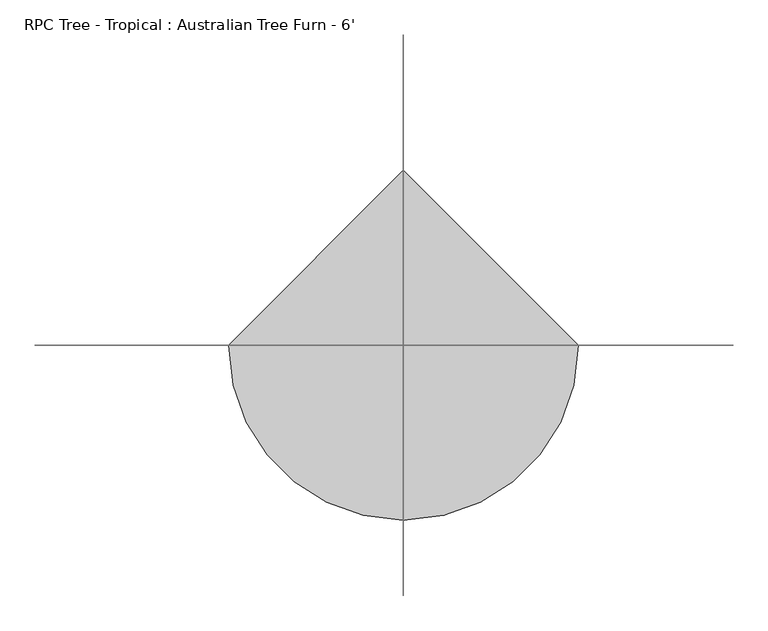
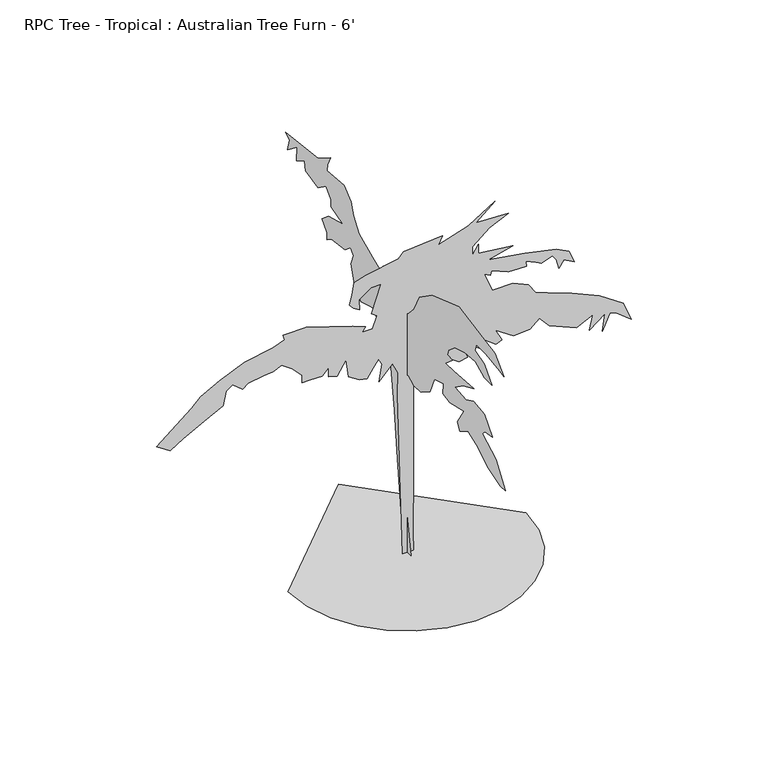
"""IFC4 building model written with IfcOpenShell, lengths in millimetres: geographic element geometry, RPC Tree - Tropical : Australian Tree Furn - 6'."""

from ifc_helpers import new_model, si_unit, origin, place, context, project, spatial, triangles, source, transform, mapped, element, save


def rpc_tree_tropical_australian_tree_furn_6_f1eb339c(model_context):
    return source(origin(), model_context, "Body", "Tessellation", [
        triangles([(-1065.0609346, 0.0, 0.0011932), (-1036.9008076, -244.0412813, 0.0011932), (-956.7128969, -468.1520205, 0.0011932), (-830.9108374, -665.916548, 0.0011932), (-665.916548, -830.9108374, 0.0011932), (-468.1520205, -956.7128969, 0.0011932), (-244.0412813, -1036.9008076, 0.0011932), (4.66e-05, -1065.0609346, 0.0011932), (244.0412813, -1036.9050224, 0.0011932), (468.1520205, -956.7128969, 0.0011932), (665.916548, -830.9108374, 0.0011932), (830.9108374, -665.916548, 0.0011932), (956.7128969, -468.1520205, 0.0011932), (1036.9008076, -244.0412813, 0.0011932), (1065.0609346, 9.31e-05, 0.0011932), (-0.0001397, 1065.0609346, 0.0011932), (783.8319523, -5.83e-05, 3048.0023254), (614.2656309, -4.97e-05, 2902.6591621), (904.9519575, -4.89e-05, 2890.5476921), (735.3856361, -4.43e-05, 2811.8202301), (583.9845577, -3.67e-05, 2684.6465973), (583.9845577, -3.2e-05, 2605.919426), (638.488789, -3.7e-05, 2690.7002975), (638.488789, -3.2e-05, 2605.919426), (947.3445734, -2.98e-05, 2569.5847252), (729.327721, -2.66e-05, 2515.0804939), (1056.3487484, -2.33e-05, 2460.5762627), (1334.9234596, -1.97e-05, 2400.0183311), (1449.9856224, -1.61e-05, 2339.4561848), (1498.4317932, -9.2e-06, 2224.394022), (1401.5393063, -1.25e-05, 2278.8982533), (1359.1466904, -8.5e-06, 2212.282552), (1334.9234596, -1.39e-05, 2303.121484), (1298.5887589, -1.68e-05, 2351.5678001), (1201.6919117, -1.47e-05, 2315.232954), (1153.2455956, -1.61e-05, 2339.4561848), (1062.4066635, -1.86e-05, 2381.8488007), (1068.4602911, -1.57e-05, 2333.4024845), (995.7908895, -1.57e-05, 2333.4024845), (904.9519575, -1.61e-05, 2339.4561848), (753.555094, -1.97e-05, 2400.0183311), (747.4971788, -1.72e-05, 2357.6257153), (692.9930202, -1.9e-05, 2387.9067158), (765.6667093, -8.5e-06, 2212.282552), (947.3445734, -8.5e-06, 2212.282552), (1086.6298216, -4.9e-06, 2151.7246204), (1147.1876804, 5e-07, 2060.8856884), (1256.196143, 3e-06, 2018.4930725), (1474.2087078, 8.1e-06, 1933.7078407), (1722.5024185, 1.46e-05, 1824.7035931), (1934.4612831, 2.32e-05, 1679.3604298), (2007.13083, 3.37e-05, 1503.7362659), (1867.8455818, 2.72e-05, 1612.7447285), (1813.3413506, 2.65e-05, 1624.8561985), (1746.7255039, 3.52e-05, 1479.5130352), (1770.9487347, 2.58e-05, 1636.9678139), (1631.6634865, 3.23e-05, 1527.9635662), (1661.944487, 2.4e-05, 1667.2488144), (1516.6013237, 2.83e-05, 1594.575198), (1274.3655281, 2.22e-05, 1697.5299603), (1183.5266687, 1.6e-05, 1800.4805077), (1098.7413643, 2.04e-05, 1727.8067459), (953.398201, 2.11e-05, 1715.6951305), (789.8898674, 1.46e-05, 1824.7035931), (850.4477262, 2.11e-05, 1715.6951305), (795.943495, 2.25e-05, 1691.4720451), (541.5961567, 1.1e-05, 1885.2615246), (699.0508627, 2.4e-05, 1667.2488144), (474.9803827, 1.46e-05, 1824.7035931), (541.5961567, 2.47e-05, 1655.1373444), (462.8688037, 2.54e-05, 1643.025729), (317.5252407, 1.93e-05, 1745.9762764), (147.9593554, 1.6e-05, 1800.4805077), (323.5814481, 2.54e-05, 1643.025729), (51.0642023, 1.86e-05, 1758.0877464), (57.1199873, 2.61e-05, 1630.9141136), (57.1199873, 5.54e-05, 1140.3804651), (57.1199873, 8.06e-05, 716.4668055), (51.0642023, 0.0001128, 177.487295), (57.1199873, 0.0001225, 0.0022127), (-39.7750749, 0.0001232, 0.0011671), (-88.22274, 3.3e-05, 1515.8520962), (-82.1665235, 2.04e-05, 1727.8067459), (-130.6141023, 1.42e-05, 1830.7572933), (-251.7328358, 2.18e-05, 1703.5836605), (-227.5092599, 1.24e-05, 1861.0382938), (-257.7890432, 9.2e-06, 1915.5425251), (-306.2361769, 1.31e-05, 1848.9266785), (-360.7395724, 1.78e-05, 1770.1993618), (-427.3553464, 1.71e-05, 1782.3109772), (-524.2521935, 1.35e-05, 1842.8689087), (-548.4753516, 3.4e-06, 2012.4351574), (-627.2027046, 1.1e-05, 1885.2615246), (-705.930094, 9.5e-06, 1909.48461), (-705.930094, 4.5e-06, 1994.2698418), (-760.4300377, 8.1e-06, 1933.7078407), (-863.3805851, 8.1e-06, 1933.7078407), (-942.1079018, 8.1e-06, 1933.7078407), (-942.1079018, 3.8e-06, 2006.3814571), (-1032.9511213, -1.7e-06, 2097.2203892), (-1123.7857658, -5.6e-06, 2163.8362358), (-1202.5131552, -3.5e-06, 2127.501535), (-1287.2984596, -3.1e-06, 2121.4436199), (-1426.5837078, -1.7e-06, 2097.2203892), (-1475.0342388, 5e-07, 2060.8856884), (-1565.8731709, -3.8e-06, 2133.55509), (-1620.3731873, -1.3e-06, 2091.1624741), (-1650.6541878, 6.3e-06, 1963.9888412), (-1820.2204365, 1.13e-05, 1879.2078243), (-2007.9562157, 1.75e-05, 1776.2572769), (-2123.0183784, 2.18e-05, 1703.5836605), (-2244.138311, 1.71e-05, 1782.3109772), (-1929.228899, 1.9e-06, 2036.6624577), (-1850.5015823, -3.1e-06, 2121.4436199), (-1680.9351883, -8.5e-06, 2212.282552), (-1456.8647083, -1.43e-05, 2309.1793991), (-1202.5131552, -1.72e-05, 2357.6257153), (-1099.5626804, -1.93e-05, 2393.960416), (-1111.6742231, -2.22e-05, 2442.4067322), (-899.7195007, -2.22e-05, 2442.4067322), (-693.8142637, -1.83e-05, 2375.7951004), (-487.9132416, -1.43e-05, 2309.1793991), (-372.8515512, -1.18e-05, 2266.7867832), (-403.1313526, -9.2e-06, 2224.394022), (-312.2919846, -9.2e-06, 2224.394022), (-269.9006222, -1.57e-05, 2333.4024845), (-318.3481919, -1.79e-05, 2369.7371853), (-233.5650312, -3.27e-05, 2618.030896), (-324.4039633, -3.27e-05, 2618.030896), (-433.4090103, -2.8e-05, 2539.303434), (-427.3553464, -2.22e-05, 2442.4067322), (-481.8595413, -2.44e-05, 2478.7457932), (-518.1942784, -2.69e-05, 2521.1341942), (-493.9711204, -3.23e-05, 2611.9731262), (-475.8016625, -3.85e-05, 2714.9275978), (-366.7957798, -4.06e-05, 2751.2625893), (-76.1107386, -4.39e-05, 2805.7668205), (-33.7189924, -4.68e-05, 2854.2129913), (317.5252407, -4.86e-05, 2884.4939919), (281.1896497, -4.43e-05, 2811.8202301), (547.6498206, -4.93e-05, 2896.6057526), (5.06e-05, -1436.4303452, 2583.0551239), (4e-05, -1222.5707245, 2617.5483673), (3.35e-05, -1077.7016602, 2617.5483673), (3.43e-05, -1050.1045801, 2548.5618805), (4.23e-05, -1201.87395, 2507.1681862), (5.12e-05, -1312.2539131, 2376.0956635), (4.59e-05, -1194.9777866, 2376.0956635), (3.77e-05, -1057.0048857, 2445.0821503), (3.1e-05, -898.3352102, 2431.2815392), (2.54e-05, -739.6697496, 2382.9917542), (2.35e-05, -643.0903976, 2300.2088711), (2.43e-05, -622.3936232, 2245.0189259), (2.8e-05, -705.1765062, 2245.0189259), (2.59e-05, -594.7965068, 2148.4395012), (3.16e-05, -725.8732807, 2155.3399521), (4.48e-05, -1036.3081112, 2176.0366539), (3.94e-05, -863.8419668, 2100.1498615), (3.65e-05, -739.6697496, 2010.4666729), (4.46e-05, -912.135894, 1996.6701313), (4.82e-05, -1029.4120205, 2051.8602219), (5.62e-05, -1194.9777866, 2031.1633747), (6.62e-05, -1326.0504547, 1893.1905464), (6.16e-05, -1208.7742556, 1872.4979141), (6.1e-05, -1167.3849215, 1831.1043652), (7.37e-05, -1374.3400944, 1713.8282387), (8.67e-05, -1526.1094643, 1506.8689236), (8.32e-05, -1443.3265812, 1499.9728329), (7.24e-05, -1243.2674263, 1562.0588688), (6.16e-05, -1070.8013546, 1665.538599), (5.44e-05, -946.6291374, 1720.7285442), (5.1e-05, -815.5523272, 1637.9414463), (4.74e-05, -781.0590837, 1706.9279331), (4.71e-05, -884.5387413, 1872.4979141), (3.89e-05, -663.7829573, 1817.3079689), (3.33e-05, -553.4071727, 1838.0046707), (3.07e-05, -560.3032997, 1934.5840954), (2.58e-05, -422.3329059, 1893.1905464), (2.74e-05, -353.3468914, 1734.5250858), (2.39e-05, -215.3743901, 1644.8417519), (1.92e-05, -104.9969069, 1637.9414463), (1.41e-05, -22.2134606, 1686.2354462), (1.13e-05, 53.6710881, 1665.538599), (7.5e-06, 88.1643133, 1741.4211765), (8.2e-06, 136.4544163, 1644.8417519), (1.16e-05, 143.3530595, 1520.6653198), (2.61e-05, 95.0629656, 1106.7508318), (4.62e-05, 32.9754059, 527.2663264), (6.56e-05, -56.7063906, 0.0011915), (6.06e-05, 60.5697358, 0.0), (5.11e-05, 88.1643133, 278.9172049), (3.29e-05, 150.2521297, 796.3117865), (1.8e-05, 198.5418056, 1224.0270309), (2.5e-06, 260.6296038, 1651.7422028), (-7.9e-06, 350.3115752, 1865.5976086), (-1.22e-05, 446.8921989, 1865.5976086), (-1.89e-05, 508.9783075, 1996.6701313), (-2.3e-05, 619.3583433, 1969.0773388), (-2.63e-05, 715.9376953, 1934.5840954), (-3.4e-05, 819.4173529, 2038.0638256), (-4.11e-05, 867.7069925, 2203.6295918), (-4.25e-05, 833.2138218, 2300.2088711), (-4.61e-05, 881.5034615, 2348.4985107), (-4.77e-05, 964.2863445, 2279.5121693), (-5.61e-05, 1171.2457323, 2251.9192314), (-5.78e-05, 1240.2321465, 2203.6295918), (-5.98e-05, 1240.2321465, 2272.6160786), (-6.6e-05, 1323.0150295, 2355.3989616), (-6.38e-05, 1219.5354446, 2438.1818447), (-5.58e-05, 998.7795879, 2500.268026), (-6.55e-05, 1178.1461105, 2555.4579712), (-6.76e-05, 1185.0422012, 2617.5483673), (-7.35e-05, 1260.9289936, 2700.331105), (-7.64e-05, 1385.1012108, 2610.6479164), (-8.63e-05, 1578.2641296, 2652.0372505), (-8.93e-05, 1592.0605259, 2734.8243484), (-9.28e-05, 1716.2371033, 2665.8378616), (-9.64e-05, 1709.3366524, 2796.910675), (-9.96e-05, 1854.2099316, 2686.5304939), (-0.0001015, 1826.6127789, 2790.0102242), (-0.0001055, 1888.703175, 2831.4036278), (-8.46e-05, 1385.1012108, 2886.5938637), (-7.97e-05, 1191.9425068, 3010.7659355), (-7.88e-05, 1233.3318409, 2921.0871071), (-7.74e-05, 1247.1325974, 2852.1006203), (-6.62e-05, 978.0828135, 2879.6934128), (-5.86e-05, 867.7069925, 2790.0102242), (-5.38e-05, 833.2138218, 2679.6344032), (-4.63e-05, 743.5305605, 2562.3584221), (-3.41e-05, 536.5754239, 2465.7747826), (-1.74e-05, 239.933665, 2348.4985107), (-2.75e-05, 377.9057485, 2479.5753937), (-1.62e-05, 191.6431533, 2382.9917542), (-3.7e-06, -1.5176088, 2251.9192314), (-2.4e-06, -104.9969069, 2362.2992672), (-3.6e-06, -187.7802351, 2527.8651787), (1.2e-06, -387.8396988, 2665.8378616), (1.54e-05, -801.7558582, 2810.706926), (3.38e-05, -1167.3849215, 2741.7204391), (4.35e-05, -1360.5435528, 2707.2271957), (5.38e-05, -1498.5165264, 2569.2545128)], [[15, 16, 1], [14, 15, 1], [14, 1, 2], [13, 14, 2], [13, 2, 3], [13, 3, 4], [12, 13, 4], [11, 12, 4], [11, 4, 5], [11, 5, 6], [11, 6, 7], [11, 7, 8], [11, 8, 9], [11, 9, 10], [141, 17, 18], [54, 55, 56], [73, 74, 75], [67, 68, 69], [24, 25, 26], [18, 19, 20], [51, 52, 53], [22, 23, 24], [84, 85, 86], [29, 30, 31], [56, 57, 58], [31, 32, 33], [130, 131, 132], [138, 139, 140], [41, 42, 43], [111, 112, 113], [110, 111, 113], [109, 110, 113], [122, 123, 124], [118, 119, 120], [18, 20, 21], [141, 18, 21], [69, 70, 71], [69, 71, 72], [28, 29, 31], [28, 31, 33], [28, 33, 34], [27, 28, 34], [27, 34, 35], [27, 35, 36], [27, 36, 37], [130, 132, 133], [130, 133, 134], [50, 51, 53], [50, 53, 54], [50, 54, 56], [50, 56, 58], [140, 141, 21], [37, 38, 39], [64, 65, 66], [64, 66, 67], [80, 81, 82], [79, 80, 82], [78, 79, 82], [77, 78, 82], [76, 77, 82], [76, 82, 83], [75, 76, 83], [97, 98, 99], [49, 50, 58], [49, 58, 59], [49, 59, 60], [48, 49, 60], [48, 60, 61], [47, 48, 61], [129, 130, 134], [129, 134, 135], [129, 135, 136], [129, 136, 137], [128, 129, 137], [108, 109, 113], [108, 113, 114], [107, 108, 114], [107, 114, 115], [106, 107, 115], [106, 115, 116], [105, 106, 116], [104, 105, 116], [103, 104, 116], [103, 116, 117], [102, 103, 117], [101, 102, 117], [101, 117, 118], [75, 83, 84], [26, 27, 37], [26, 37, 39], [26, 39, 40], [26, 40, 41], [26, 41, 43], [92, 93, 94], [92, 94, 95], [126, 127, 128], [101, 118, 120], [100, 101, 120], [100, 120, 121], [99, 100, 121], [97, 99, 121], [96, 97, 121], [95, 96, 121], [95, 121, 122], [92, 95, 122], [92, 122, 124], [140, 21, 22], [88, 89, 90], [24, 26, 43], [22, 24, 43], [88, 90, 91], [88, 91, 92], [88, 92, 124], [87, 88, 124], [87, 124, 125], [47, 61, 62], [47, 62, 63], [47, 63, 64], [46, 47, 64], [45, 46, 64], [44, 45, 64], [44, 64, 67], [43, 44, 67], [137, 138, 140], [128, 137, 140], [126, 128, 140], [126, 140, 22], [126, 22, 43], [126, 43, 67], [126, 67, 69], [126, 69, 72], [126, 72, 73], [125, 126, 73], [87, 125, 73], [87, 73, 75], [87, 75, 84], [87, 84, 86], [231, 232, 233], [156, 157, 158], [240, 241, 142], [222, 223, 224], [218, 219, 220], [220, 221, 222], [218, 220, 222], [153, 154, 155], [240, 142, 143], [239, 240, 143], [146, 147, 148], [205, 206, 207], [162, 163, 164], [156, 158, 159], [216, 217, 218], [216, 218, 222], [166, 167, 168], [166, 168, 169], [222, 224, 225], [239, 143, 144], [238, 239, 144], [146, 148, 149], [145, 146, 149], [165, 166, 169], [165, 169, 170], [207, 208, 209], [188, 189, 190], [188, 190, 191], [188, 191, 192], [187, 188, 192], [187, 192, 193], [186, 187, 193], [186, 193, 194], [185, 186, 194], [171, 172, 173], [171, 173, 174], [145, 149, 150], [155, 156, 159], [165, 170, 171], [165, 171, 174], [175, 176, 177], [182, 183, 184], [205, 207, 209], [205, 209, 210], [204, 205, 210], [203, 204, 210], [161, 162, 164], [161, 164, 165], [161, 165, 174], [160, 161, 174], [159, 160, 174], [159, 174, 175], [159, 175, 177], [155, 159, 177], [238, 144, 145], [238, 145, 150], [237, 238, 150], [237, 150, 151], [237, 151, 152], [236, 237, 152], [235, 236, 152], [235, 152, 153], [235, 153, 155], [235, 155, 177], [235, 177, 178], [234, 235, 178], [234, 178, 179], [234, 179, 180], [234, 180, 181], [234, 181, 182], [234, 182, 184], [231, 233, 234], [231, 234, 184], [214, 215, 216], [214, 216, 222], [213, 214, 222], [213, 222, 225], [213, 225, 226], [212, 213, 226], [212, 226, 227], [212, 227, 228], [211, 212, 228], [210, 211, 228], [210, 228, 229], [203, 210, 229], [203, 229, 230], [202, 203, 230], [184, 185, 194], [184, 194, 195], [231, 184, 195], [230, 231, 195], [230, 195, 196], [230, 196, 197], [202, 230, 197], [202, 197, 198], [201, 202, 198], [200, 201, 198], [199, 200, 198]], closed=False),
    ])


if __name__ == "__main__":
    model = new_model("IFC4")
    model_context = context("Model", 3, world=origin())
    ifc_project = project(units=[si_unit("LENGTHUNIT", "METRE", prefix="MILLI")], contexts=[model_context])
    site = spatial("IfcSite", under=ifc_project)
    building = spatial("IfcBuilding", under=site)
    placement = place(None, origin())
    rpc_tree_tropical_australian_tree_furn_6_shape = rpc_tree_tropical_australian_tree_furn_6_f1eb339c(model_context)
    element("IfcGeographicElement", 1, ObjectType="RPC Tree - Tropical : Australian Tree Furn - 6'", at=placement, inside=building, context=model_context, shape_type="MappedRepresentation", body=[
        mapped(rpc_tree_tropical_australian_tree_furn_6_shape, transform((0.0, 0.0, 0.0), x_axis=(1.0, 0.0, 0.0), y_axis=(0.0, 1.0, 0.0), z_axis=(0.0, 0.0, 1.0))),
    ])
    save(model, "model.ifc")

# Revit data of these elements
# Type "RPC Tree - Tropical : Australian Tree Furn - 6'"
#   built-in parameter 1005198 = "{2, 15},{39, RPC-16-FVCN-UWG0-AP53-A000-ST1L-LVER-AU},{1, 0},{1, 0},{2, 13},{1, 8},{5, Color},{1, 0},{1, 0},{3, 0.8},{3, 0.8},{3, 0.8},{1, 8},{7, BBoxMin},{1, 0},{1, 0},{1, 0},{1, 0},{1, 0},{1, 8},{7, BBoxMax},{1, 0},{1, 0},{1, 0},{1, 0},{1, 0},{2, 11},{9, RPCTypeId},{1, 0},{1, 0},{39, RPC-16-FVCN-UWG0-AP53-A000-ST1L-LVER-AU},{1, 6},{14, RPCPlantHeight},{1, 0},{1, 0},{1, 6},{2, 11},{7, keyword},{1, 0},{1, 0},{35, :RPCs:Trees [Tropical]:Geometry:RPC},{2, 11},{8, category},{1, 0},{1, 0},{16, Trees [Tropical]},{2, 11},{12, LocalizedUID},{1, 0},{1, 0},{20, Australian Tree Fern},{2, 14},{6, Height},{1, 0},{1, 0},{1, 6},{1, 2},{16, Cast Reflections},{1, 0},{1, 0},{1, 0},{1, 2},{12, Cast Shadows},{1, 0},{1, 0},{1, 1},{1, 2},{9, Lock View},{1, 0},{1, 0},{1, 0},{1, 4},{5, ViewC},{1, 0},{1, 0},{1, 0},{21, assetlibrary_base.fbx},{1, 5},"
#   built-in parameter 1005195 = "RPC-16-FVCN-UWG0-AP53-A000-ST1L-LVER-AU"
#   Type Comments = "Australian Tree Furn"
#   Assembly Code = "G2050500"
#   Height = 10' - 0"
#   Plan Symbol = element 352425
#   Default Elevation = 0
